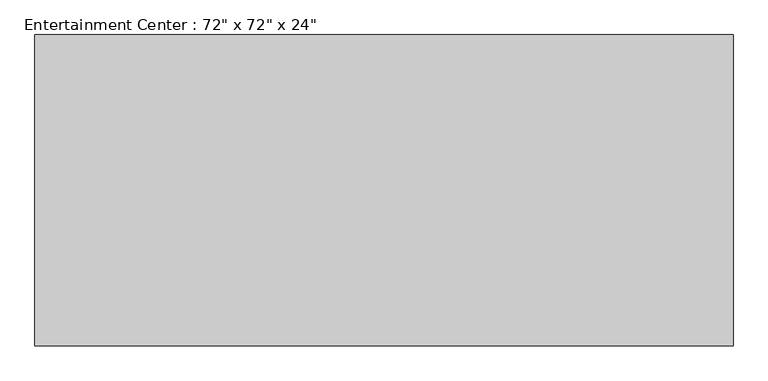
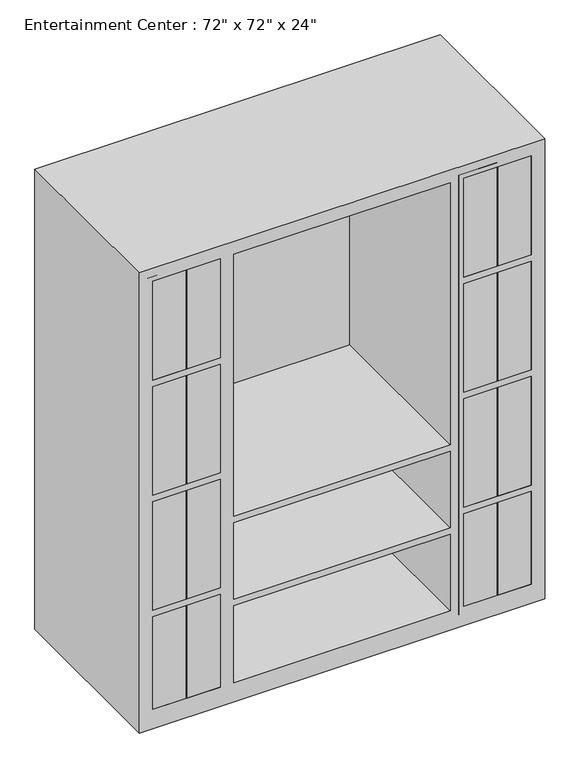
"""IFC4 building model written with IfcOpenShell, lengths in millimetres: furniture geometry."""

from ifc_helpers import new_model, si_unit, point, frame, frame_2d, origin, place, context, project, spatial, polyline, circle_curve, trimmed, segment, composite_curve, outline, extrude, faceted_brep, source, transform, mapped, element, save


def furniture_cdca18a6(model_context):
    return source(origin(), model_context, "Body", "SolidModel", [
        faceted_brep([(762.0, -781.05, 0.0), (762.0, -781.05, 1828.8), (-762.0, -781.05, 1828.8), (-762.0, -781.05, 0.0), (-457.2, -781.05, 1778.0), (-457.2, -781.05, 1384.3), (-711.2, -781.05, 1384.3), (-711.2, -781.05, 1778.0), (-457.2, -781.05, 76.2), (-711.2, -781.05, 76.2), (-711.2, -781.05, 444.5), (-457.2, -781.05, 444.5), (711.2, -781.05, 1384.3), (457.2, -781.05, 1384.3), (457.2, -781.05, 1778.0), (711.2, -781.05, 1778.0), (-406.4, -781.05, 736.6), (-406.4, -781.05, 1778.0), (406.4, -781.05, 1778.0), (406.4, -781.05, 736.6), (406.4, -781.05, 76.2), (-406.4, -781.05, 76.2), (-406.4, -781.05, 381.0), (406.4, -781.05, 381.0), (711.2, -781.05, 76.2), (457.2, -781.05, 76.2), (457.2, -781.05, 444.5), (711.2, -781.05, 444.5), (-711.2, -781.05, 469.9), (-711.2, -781.05, 901.7), (-457.2, -781.05, 901.7), (-457.2, -781.05, 469.9), (-457.2, -781.05, 1358.9), (-457.2, -781.05, 927.1), (-711.2, -781.05, 927.1), (-711.2, -781.05, 1358.9), (457.2, -781.05, 1358.9), (711.2, -781.05, 1358.9), (711.2, -781.05, 927.1), (457.2, -781.05, 927.1), (457.2, -781.05, 901.7), (711.2, -781.05, 901.7), (711.2, -781.05, 469.9), (457.2, -781.05, 469.9), (406.4, -781.05, 406.4), (-406.4, -781.05, 406.4), (-406.4, -781.05, 711.2), (406.4, -781.05, 711.2), (762.0, -101.6, 0.0), (-762.0, -101.6, 0.0), (-762.0, -101.6, 1828.8), (762.0, -101.6, 1828.8), (-457.2, -127.0, 1778.0), (-457.2, -127.0, 1384.3), (-711.2, -127.0, 1384.3), (-711.2, -127.0, 1778.0), (-457.2, -127.0, 76.2), (-711.2, -127.0, 76.2), (-711.2, -127.0, 444.5), (-457.2, -127.0, 444.5), (711.2, -127.0, 1384.3), (457.2, -127.0, 1384.3), (457.2, -127.0, 1778.0), (711.2, -127.0, 1778.0), (-406.4, -127.0, 736.6), (-406.4, -127.0, 1778.0), (406.4, -127.0, 1778.0), (406.4, -127.0, 736.6), (406.4, -127.0, 76.2), (-406.4, -127.0, 76.2), (-406.4, -127.0, 381.0), (406.4, -127.0, 381.0), (711.2, -127.0, 76.2), (457.2, -127.0, 76.2), (457.2, -127.0, 444.5), (711.2, -127.0, 444.5), (-711.2, -127.0, 469.9), (-711.2, -127.0, 901.7), (-457.2, -127.0, 901.7), (-457.2, -127.0, 469.9), (-457.2, -127.0, 1358.9), (-457.2, -127.0, 927.1), (-711.2, -127.0, 927.1), (-711.2, -127.0, 1358.9), (457.2, -127.0, 1358.9), (711.2, -127.0, 1358.9), (711.2, -127.0, 927.1), (457.2, -127.0, 927.1), (457.2, -127.0, 901.7), (711.2, -127.0, 901.7), (711.2, -127.0, 469.9), (457.2, -127.0, 469.9), (406.4, -127.0, 406.4), (-406.4, -127.0, 406.4), (-406.4, -127.0, 711.2), (406.4, -127.0, 711.2)], [[[0, 1, 2, 3], [4, 5, 6, 7], [8, 9, 10, 11], [12, 13, 14, 15], [16, 17, 18, 19], [20, 21, 22, 23], [24, 25, 26, 27], [28, 29, 30, 31], [32, 33, 34, 35], [36, 37, 38, 39], [40, 41, 42, 43], [44, 45, 46, 47]], [[48, 49, 50, 51]], [[1, 0, 48, 51]], [[2, 1, 51, 50]], [[3, 2, 50, 49]], [[0, 3, 49, 48]], [[5, 4, 52, 53]], [[6, 5, 53, 54]], [[7, 6, 54, 55]], [[4, 7, 55, 52]], [[9, 8, 56, 57]], [[10, 9, 57, 58]], [[11, 10, 58, 59]], [[8, 11, 59, 56]], [[13, 12, 60, 61]], [[14, 13, 61, 62]], [[15, 14, 62, 63]], [[12, 15, 63, 60]], [[17, 16, 64, 65]], [[18, 17, 65, 66]], [[19, 18, 66, 67]], [[16, 19, 67, 64]], [[21, 20, 68, 69]], [[22, 21, 69, 70]], [[23, 22, 70, 71]], [[20, 23, 71, 68]], [[25, 24, 72, 73]], [[26, 25, 73, 74]], [[27, 26, 74, 75]], [[24, 27, 75, 72]], [[29, 28, 76, 77]], [[30, 29, 77, 78]], [[31, 30, 78, 79]], [[28, 31, 79, 76]], [[33, 32, 80, 81]], [[34, 33, 81, 82]], [[35, 34, 82, 83]], [[32, 35, 83, 80]], [[37, 36, 84, 85]], [[38, 37, 85, 86]], [[39, 38, 86, 87]], [[36, 39, 87, 84]], [[41, 40, 88, 89]], [[42, 41, 89, 90]], [[43, 42, 90, 91]], [[40, 43, 91, 88]], [[45, 44, 92, 93]], [[46, 45, 93, 94]], [[47, 46, 94, 95]], [[44, 47, 95, 92]], [[53, 52, 55, 54]], [[57, 56, 59, 58]], [[61, 60, 63, 62]], [[65, 64, 67, 66]], [[69, 68, 71, 70]], [[73, 72, 75, 74]], [[77, 76, 79, 78]], [[81, 80, 83, 82]], [[85, 84, 87, 86]], [[89, 88, 91, 90]], [[93, 92, 95, 94]]]),
        extrude(outline(composite_curve([segment(polyline([(1003.3, -556.7986452), (1003.3, -581.025), (825.5, -581.025), (825.5, -556.7986452)]), True, "CONTINUOUS"), segment(trimmed(circle_curve(frame_2d((850.9, -556.7986452)), 25.4), [point((825.5, -556.7986452))], [point((850.9, -531.3986452))], False, "CARTESIAN"), True, "CONTINUOUS"), segment(polyline([(850.9, -531.3986452), (977.9, -531.3986452)]), True, "CONTINUOUS"), segment(trimmed(circle_curve(frame_2d((977.9, -556.7986452)), 25.4), [point((977.9, -531.3986452))], [point((1003.3, -556.7986452))], False, "CARTESIAN"), True, "CONTINUOUS")], self_intersect=False)), frame((0.0, -714.375, 0.0), z_axis=(0.0, 1.0, 0.0), x_axis=(0.0, 0.0, 1.0)), (0.0, 0.0, 1.0), 3.175),
        extrude(outline(composite_curve([segment(trimmed(circle_curve(frame_2d((977.9, -611.98125)), 25.4), [point((1003.3, -611.98125))], [point((977.9, -637.38125))], False, "CARTESIAN"), True, "CONTINUOUS"), segment(polyline([(977.9, -637.38125), (850.9, -637.38125)]), True, "CONTINUOUS"), segment(trimmed(circle_curve(frame_2d((850.9, -611.98125)), 25.4), [point((850.9, -637.38125))], [point((825.5, -611.98125))], False, "CARTESIAN"), True, "CONTINUOUS"), segment(polyline([(825.5, -611.98125), (825.5, -587.375), (1003.3, -587.375), (1003.3, -611.98125)]), True, "CONTINUOUS")], self_intersect=False)), frame((0.0, -714.375, 0.0), z_axis=(0.0, 1.0, 0.0), x_axis=(0.0, 0.0, 1.0)), (0.0, 0.0, 1.0), 3.175),
        extrude(outline(composite_curve([segment(trimmed(circle_curve(frame_2d((977.9, 556.7986452)), 25.4), [point((1003.3, 556.7986452))], [point((977.9, 531.3986452))], False, "CARTESIAN"), True, "CONTINUOUS"), segment(polyline([(977.9, 531.3986452), (850.9, 531.3986452)]), True, "CONTINUOUS"), segment(trimmed(circle_curve(frame_2d((850.9, 556.7986452)), 25.4), [point((850.9, 531.3986452))], [point((825.5, 556.7986452))], False, "CARTESIAN"), True, "CONTINUOUS"), segment(polyline([(825.5, 556.7986452), (825.5, 581.025), (1003.3, 581.025), (1003.3, 556.7986452)]), True, "CONTINUOUS")], self_intersect=False)), frame((0.0, -714.375, 0.0), z_axis=(0.0, 1.0, 0.0), x_axis=(0.0, 0.0, 1.0)), (0.0, 0.0, 1.0), 3.175),
        extrude(outline(composite_curve([segment(polyline([(1003.3, 611.98125), (1003.3, 587.375), (825.5, 587.375), (825.5, 611.98125)]), True, "CONTINUOUS"), segment(trimmed(circle_curve(frame_2d((850.9, 611.98125)), 25.4), [point((825.5, 611.98125))], [point((850.9, 637.38125))], False, "CARTESIAN"), True, "CONTINUOUS"), segment(polyline([(850.9, 637.38125), (977.9, 637.38125)]), True, "CONTINUOUS"), segment(trimmed(circle_curve(frame_2d((977.9, 611.98125)), 25.4), [point((977.9, 637.38125))], [point((1003.3, 611.98125))], False, "CARTESIAN"), True, "CONTINUOUS")], self_intersect=False)), frame((0.0, -714.375, 0.0), z_axis=(0.0, 1.0, 0.0), x_axis=(0.0, 0.0, 1.0)), (0.0, 0.0, 1.0), 3.175),
        extrude(outline(polyline([(-730.25, -711.2), (-587.375, -711.2), (-587.375, -781.05), (-730.25, -781.05), (-730.25, -711.2)])), frame((0.0, 0.0, 50.8), z_axis=(0.0, 0.0, 1.0), x_axis=(1.0, 0.0, 0.0)), (0.0, 0.0, 1.0), 1746.25),
        extrude(outline(polyline([(-581.025, -711.2), (-438.15, -711.2), (-438.15, -781.05), (-581.025, -781.05), (-581.025, -711.2)])), frame((0.0, 0.0, 50.8), z_axis=(0.0, 0.0, 1.0), x_axis=(1.0, 0.0, 0.0)), (0.0, 0.0, 1.0), 1746.25),
        extrude(outline(polyline([(587.375, -711.2), (730.25, -711.2), (730.25, -781.05), (587.375, -781.05), (587.375, -711.2)])), frame((0.0, 0.0, 50.8), z_axis=(0.0, 0.0, 1.0), x_axis=(1.0, 0.0, 0.0)), (0.0, 0.0, 1.0), 1746.25),
        extrude(outline(polyline([(438.15, -711.2), (581.025, -711.2), (581.025, -781.05), (438.15, -781.05), (438.15, -711.2)])), frame((0.0, 0.0, 50.8), z_axis=(0.0, 0.0, 1.0), x_axis=(1.0, 0.0, 0.0)), (0.0, 0.0, 1.0), 1746.25),
    ])


if __name__ == "__main__":
    model = new_model("IFC4")
    model_context = context("Model", 3, world=origin())
    ifc_project = project(units=[si_unit("LENGTHUNIT", "METRE", prefix="MILLI")], contexts=[model_context])
    site = spatial("IfcSite", under=ifc_project)
    building = spatial("IfcBuilding", under=site)
    placement = place(None, origin())
    furniture_shape = furniture_cdca18a6(model_context)
    element("IfcFurniture", 1, ObjectType="Entertainment Center : 72\" x 72\" x 24\"", at=placement, inside=building, context=model_context, shape_type="MappedRepresentation", body=[
        mapped(furniture_shape, transform((0.0, 0.0, 0.0), x_axis=(1.0, 0.0, 0.0), y_axis=(0.0, 1.0, 0.0), z_axis=(0.0, 0.0, 1.0))),
    ])
    save(model, "model.ifc")

# Revit data of these elements
# Type "Entertainment Center : 72\" x 72\" x 24\""
#   Assembly Code = "E2020200"
#   Center Width = 2' - 8"
#   Depth = 2' - 0"
#   Height = 6' - 0"
#   Width = 5' - 0"
#   Material = none
#   Default Elevation = 0
# Element 1 (IfcFurniture, "Entertainment Center : 72\" x 72\" x 24\"")
#   Materials on its faces: "Steel, Chrome Plated", "Glass - Clear, Grey"
# Materials
#   "Steel, Chrome Plated": class "Metal", colour RGB 17 17 17, transparency 0, Description = "Chromiuim plated steel", Cost = 0
#   "Glass - Clear, Grey": class "Glass", colour RGB 252 255 255, transparency 0.64
